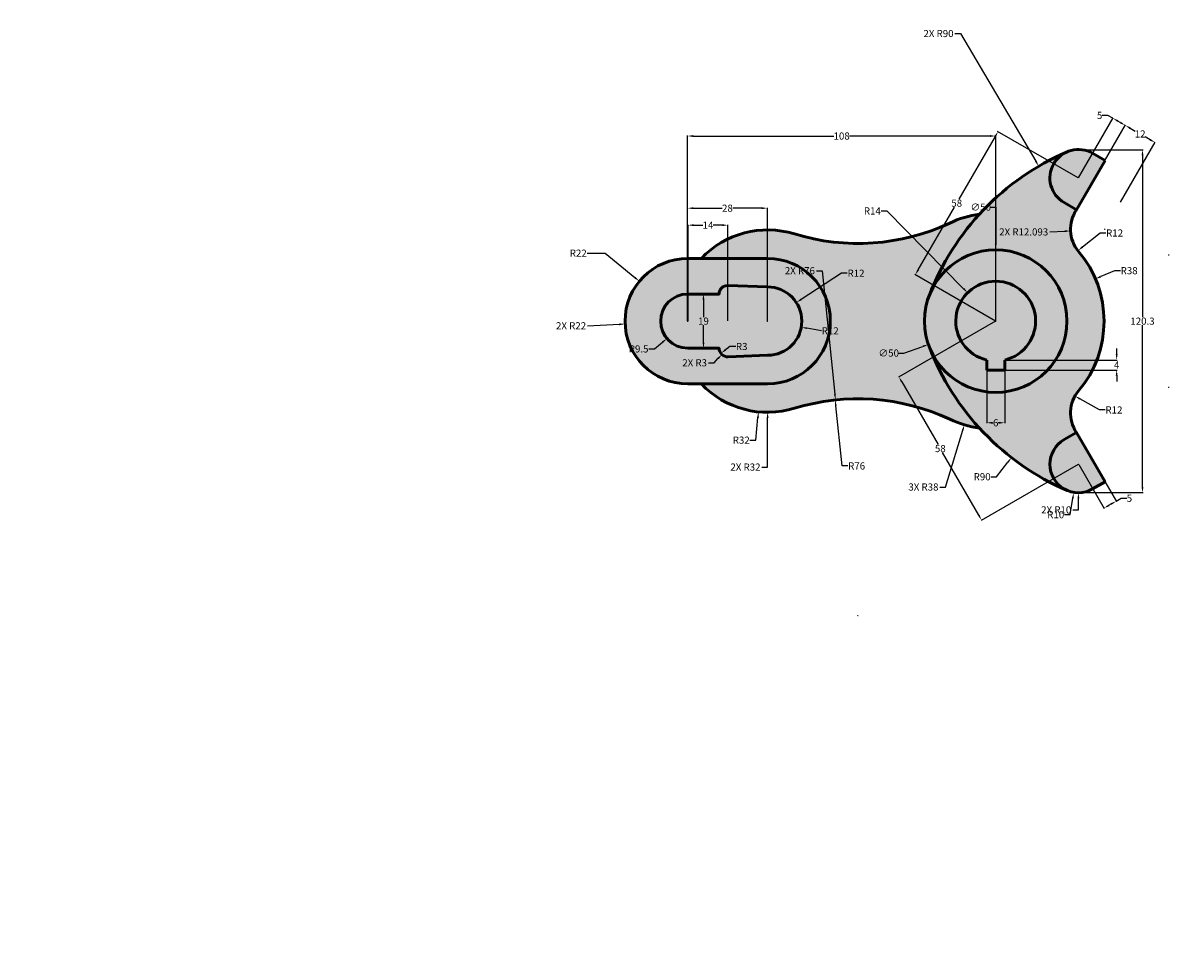
# Model space of a CAD drawing. Units: millimetres. Extents: x -3 to 399, y -3 to 324.
import ezdxf

# ---------------------------------------------------------------- set-up
doc = ezdxf.new("R2010")
doc.units = ezdxf.units.MM
doc.header["$MEASUREMENT"] = 0
for name, color, linetype, lineweight in [('Dimension', 120, 'Continuous', 25), ('M-CONS', 8, 'Continuous', 13), ('M-OUTL', 1, 'Continuous', 50)]:
    doc.layers.add(name, color=color, linetype=linetype, lineweight=lineweight)
doc.layers.add('M-HATC', color=9, linetype='Continuous', lineweight=18, true_color=0xc7c8ca)
doc.styles.get("Standard").update_dxf_attribs({"font": 'arial.ttf'})
doc.dimstyles.get("Standard").update_dxf_attribs({"dimtxt": 2.5, "dimasz": 2, "dimexe": 0.18, "dimexo": 0.0625, "dimgap": 0.09, "dimtad": 0, "dimtih": 1, "dimtoh": 1, "dimdec": 0, "dimzin": 0, "dimdsep": 46, "dimtxsty": 'Standard', "dimcen": 0.09, "dimadec": 0, "dimazin": 0, "dimtfac": 1, "dimtdec": 0, "dimtofl": 0, "dimtmove": 0, "dimatfit": 3, "dimfxl": 1, "dimtolj": 1, "dimtzin": 0, "dimarcsym": 0})

# ---------------------------------------------------------------- blocks, each defined once
blk = doc.blocks.new('*D1')
at = {"layer": 'Defpoints', "color": 0, "transparency": 16777216}
for p in [(213.19, 233.77), (230.17, 219.78)]:
    blk.add_point(p, dxfattribs=at)
at = {"layer": 'Dimension', "color": 0, "lineweight": -2, "transparency": 16777216}
for p, q in [((194.83, 243.63), (201.21, 243.63)), ((201.21, 243.63), (211.64, 235.04)), ((230.08, 219.78), (230.26, 219.78)), ((230.17, 219.69), (230.17, 219.87))]:
    blk.add_line(p, q, dxfattribs=at)
at = {"layer": 'Dimension', "color": 0, "transparency": 16777216}
blk.add_solid([(211.86, 235.3), (211.43, 234.78), (213.19, 233.77)], dxfattribs=at)
at = {"layer": 'Dimension', "color": 0, "transparency": 16777216, "insert": (191.77, 243.63), "char_height": 2.5, "attachment_point": 5}
blk.add_mtext('\\A1;R22', dxfattribs=at)
blk = doc.blocks.new('*D2')
at = {"layer": 'Defpoints', "color": 0, "transparency": 16777216}
for p in [(235.67, 229.28), (235.67, 210.28), (235.67, 210.28)]:
    blk.add_point(p, dxfattribs=at)
at = {"layer": 'Dimension', "color": 0, "lineweight": -2, "transparency": 16777216}
for p, q in [((235.73, 229.28), (235.85, 229.28)), ((235.67, 227.28), (235.67, 221.15)), ((235.67, 212.28), (235.67, 218.41)), ((235.73, 210.28), (235.85, 210.28))]:
    blk.add_line(p, q, dxfattribs=at)
at = {"layer": 'Dimension', "color": 0, "transparency": 16777216}
for points in [[(235.34, 227.28), (236, 227.28), (235.67, 229.28)], [(235.34, 212.28), (236, 212.28), (235.67, 210.28)]]:
    blk.add_solid(points, dxfattribs=at)
at = {"layer": 'Dimension', "color": 0, "transparency": 16777216, "insert": (235.67, 219.78), "char_height": 2.5, "attachment_point": 5}
blk.add_mtext('\\A1;19', dxfattribs=at)
blk = doc.blocks.new('*D3')
at = {"layer": 'Defpoints', "color": 0, "transparency": 16777216}
for p in [(244.17, 210.28), (241.76, 208.49)]:
    blk.add_point(p, dxfattribs=at)
at = {"layer": 'Dimension', "color": 0, "lineweight": -2, "transparency": 16777216}
for p, q in [((244.97, 210.88), (243.37, 209.68)), ((246.97, 210.88), (244.97, 210.88))]:
    blk.add_line(p, q, dxfattribs=at)
at = {"layer": 'Dimension', "color": 0, "transparency": 16777216}
blk.add_solid([(243.17, 209.95), (243.57, 209.42), (241.76, 208.49)], dxfattribs=at)
at = {"layer": 'Dimension', "color": 0, "transparency": 16777216, "insert": (249.08, 210.88), "char_height": 2.5, "attachment_point": 5}
blk.add_mtext('\\A1;R3', dxfattribs=at)
blk = doc.blocks.new('*D4')
at = {"layer": 'Defpoints', "color": 0, "transparency": 16777216}
for p in [(258.17, 219.78), (254.98, 187.94)]:
    blk.add_point(p, dxfattribs=at)
at = {"layer": 'Dimension', "color": 0, "lineweight": -2, "transparency": 16777216}
for p, q in [((258.08, 219.78), (258.26, 219.78)), ((258.17, 219.69), (258.17, 219.87)), ((253.99, 178.03), (254.78, 185.95)), ((251.99, 178.03), (253.99, 178.03))]:
    blk.add_line(p, q, dxfattribs=at)
at = {"layer": 'Dimension', "color": 0, "transparency": 16777216}
blk.add_solid([(254.45, 185.98), (255.12, 185.92), (254.98, 187.94)], dxfattribs=at)
at = {"layer": 'Dimension', "color": 0, "transparency": 16777216, "insert": (248.93, 178.03), "char_height": 2.5, "attachment_point": 5}
blk.add_mtext('\\A1;R32', dxfattribs=at)
blk = doc.blocks.new('*D5')
at = {"layer": 'Defpoints', "color": 0, "transparency": 16777216}
for p in [(258.08, 259.41), (230.08, 219.78), (258.08, 219.78)]:
    blk.add_point(p, dxfattribs=at)
at = {"layer": 'Dimension', "color": 0, "lineweight": -2, "transparency": 16777216}
for p, q in [((230.08, 219.84), (230.08, 259.59)), ((232.08, 259.41), (242.18, 259.41)), ((256.08, 259.41), (245.98, 259.41)), ((258.08, 219.84), (258.08, 259.59))]:
    blk.add_line(p, q, dxfattribs=at)
at = {"layer": 'Dimension', "color": 0, "transparency": 16777216}
for points in [[(232.08, 259.74), (232.08, 259.07), (230.08, 259.41)], [(256.08, 259.74), (256.08, 259.07), (258.08, 259.41)]]:
    blk.add_solid(points, dxfattribs=at)
at = {"layer": 'Dimension', "color": 0, "transparency": 16777216, "insert": (244.08, 259.41), "char_height": 2.5, "attachment_point": 5}
blk.add_mtext('\\A1;28', dxfattribs=at)
blk = doc.blocks.new('*D6')
at = {"layer": 'Defpoints', "color": 0, "transparency": 16777216}
for p in [(244.26, 253.44), (230.26, 219.78), (244.26, 219.78)]:
    blk.add_point(p, dxfattribs=at)
at = {"layer": 'Dimension', "color": 0, "lineweight": -2, "transparency": 16777216}
for p, q in [((230.26, 219.84), (230.26, 253.62)), ((232.26, 253.44), (235.5, 253.44)), ((242.26, 253.44), (239.02, 253.44)), ((244.26, 219.84), (244.26, 253.62))]:
    blk.add_line(p, q, dxfattribs=at)
at = {"layer": 'Dimension', "color": 0, "transparency": 16777216}
for points in [[(232.26, 253.78), (232.26, 253.11), (230.26, 253.44)], [(242.26, 253.78), (242.26, 253.11), (244.26, 253.44)]]:
    blk.add_solid(points, dxfattribs=at)
at = {"layer": 'Dimension', "color": 0, "transparency": 16777216, "insert": (237.26, 253.44), "char_height": 2.5, "attachment_point": 5}
blk.add_mtext('\\A1;14', dxfattribs=at)
blk = doc.blocks.new('*D7')
at = {"layer": 'Defpoints', "color": 0, "transparency": 16777216}
for p in [(338.17, 284.73), (230.08, 219.78), (338.17, 219.78)]:
    blk.add_point(p, dxfattribs=at)
at = {"layer": 'Dimension', "color": 0, "lineweight": -2, "transparency": 16777216}
for p, q in [((230.08, 219.84), (230.08, 284.91)), ((232.08, 284.73), (281.39, 284.73)), ((336.17, 284.73), (286.86, 284.73)), ((338.17, 219.84), (338.17, 284.91))]:
    blk.add_line(p, q, dxfattribs=at)
at = {"layer": 'Dimension', "color": 0, "transparency": 16777216}
for points in [[(232.08, 285.07), (232.08, 284.4), (230.08, 284.73)], [(336.17, 285.07), (336.17, 284.4), (338.17, 284.73)]]:
    blk.add_solid(points, dxfattribs=at)
at = {"layer": 'Dimension', "color": 0, "transparency": 16777216, "insert": (284.13, 284.73), "char_height": 2.5, "attachment_point": 5}
blk.add_mtext('\\A1;108', dxfattribs=at)
blk = doc.blocks.new('*D8')
at = {"layer": 'Defpoints', "color": 0, "transparency": 16777216}
for p in [(338.99, 286.28), (367.17, 270.01), (338.17, 219.78)]:
    blk.add_point(p, dxfattribs=at)
at = {"layer": 'Dimension', "color": 0, "lineweight": -2, "transparency": 16777216}
for p, q in [((367.12, 270.04), (338.83, 286.37)), ((337.99, 284.55), (325.28, 262.53)), ((310.99, 237.78), (323.7, 259.8)), ((338.12, 219.81), (309.83, 236.14))]:
    blk.add_line(p, q, dxfattribs=at)
at = {"layer": 'Dimension', "color": 0, "transparency": 16777216}
for points in [[(337.7, 284.72), (338.28, 284.38), (338.99, 286.28)], [(310.7, 237.95), (311.28, 237.62), (309.99, 236.05)]]:
    blk.add_solid(points, dxfattribs=at)
at = {"layer": 'Dimension', "color": 0, "transparency": 16777216, "insert": (324.49, 261.17), "char_height": 2.5, "attachment_point": 5}
blk.add_mtext('\\A1;58', dxfattribs=at)
blk = doc.blocks.new('*D9')
at = {"layer": 'Defpoints', "color": 0, "transparency": 16777216}
for p in [(281.87, 192.11), (289.85, 116.53)]:
    blk.add_point(p, dxfattribs=at)
at = {"layer": 'Dimension', "color": 0, "lineweight": -2, "transparency": 16777216}
for p, q in [((284.31, 168.97), (282.08, 190.12)), ((286.31, 168.97), (284.31, 168.97))]:
    blk.add_line(p, q, dxfattribs=at)
at = {"layer": 'Dimension', "color": 0, "transparency": 16777216}
blk.add_solid([(282.41, 190.16), (281.75, 190.09), (281.87, 192.11)], dxfattribs=at)
at = {"layer": 'Dimension', "color": 0, "transparency": 16777216, "insert": (289.39, 168.97), "char_height": 2.5, "attachment_point": 5}
blk.add_mtext('\\A1;R76', dxfattribs=at)
blk = doc.blocks.new('*D10')
at = {"layer": 'Defpoints', "color": 0, "transparency": 16777216}
for p in [(338.17, 219.78), (367.17, 169.55), (333.23, 149.95)]:
    blk.add_point(p, dxfattribs=at)
at = {"layer": 'Dimension', "color": 0, "lineweight": -2, "transparency": 16777216}
for p, q in [((338.12, 219.75), (304.07, 200.09)), ((305.23, 198.45), (317.94, 176.44)), ((332.23, 151.69), (319.51, 173.7)), ((367.12, 169.52), (333.07, 149.86))]:
    blk.add_line(p, q, dxfattribs=at)
at = {"layer": 'Dimension', "color": 0, "transparency": 16777216}
for points in [[(305.51, 198.62), (304.94, 198.29), (304.23, 200.18)], [(332.51, 151.85), (331.94, 151.52), (333.23, 149.95)]]:
    blk.add_solid(points, dxfattribs=at)
at = {"layer": 'Dimension', "color": 0, "transparency": 16777216, "insert": (318.73, 175.07), "char_height": 2.5, "attachment_point": 5}
blk.add_mtext('\\A1;58', dxfattribs=at)
blk = doc.blocks.new('*D11')
at = {"layer": 'Defpoints', "color": 0, "transparency": 16777216}
for p in [(398.88, 243), (343.69, 171.91)]:
    blk.add_point(p, dxfattribs=at)
at = {"layer": 'Dimension', "color": 0, "lineweight": -2, "transparency": 16777216}
for p, q in [((398.79, 243), (398.97, 243)), ((398.88, 242.91), (398.88, 243.09)), ((338.48, 165.19), (342.47, 170.33)), ((336.48, 165.19), (338.48, 165.19))]:
    blk.add_line(p, q, dxfattribs=at)
at = {"layer": 'Dimension', "color": 0, "transparency": 16777216}
blk.add_solid([(342.2, 170.53), (342.73, 170.12), (343.69, 171.91)], dxfattribs=at)
at = {"layer": 'Dimension', "color": 0, "transparency": 16777216, "insert": (333.41, 165.19), "char_height": 2.5, "attachment_point": 5}
blk.add_mtext('\\A1;R90', dxfattribs=at)
blk = doc.blocks.new('*D12')
at = {"layer": 'Defpoints', "color": 0, "transparency": 16777216}
for p in [(361.79, 227.98), (314.55, 211.59)]:
    blk.add_point(p, dxfattribs=at)
at = {"layer": 'Dimension', "color": 0, "lineweight": -2, "transparency": 16777216}
for p, q in [((338.08, 219.78), (338.26, 219.78)), ((338.17, 219.69), (338.17, 219.87)), ((305.89, 208.58), (312.66, 210.93)), ((303.89, 208.58), (305.89, 208.58))]:
    blk.add_line(p, q, dxfattribs=at)
at = {"layer": 'Dimension', "color": 0, "transparency": 16777216}
blk.add_solid([(312.55, 211.24), (312.77, 210.62), (314.55, 211.59)], dxfattribs=at)
at = {"layer": 'Dimension', "color": 0, "transparency": 16777216, "insert": (300.65, 208.58), "char_height": 2.5, "attachment_point": 5}
blk.add_mtext('\\A1;∅50', dxfattribs=at)
blk = doc.blocks.new('*D13')
at = {"layer": 'Defpoints', "color": 0, "transparency": 16777216}
for p in [(268.24, 226.31), (258.17, 219.78)]:
    blk.add_point(p, dxfattribs=at)
at = {"layer": 'Dimension', "color": 0, "lineweight": -2, "transparency": 16777216}
for p, q in [((284.11, 236.59), (269.92, 227.39)), ((286.11, 236.59), (284.11, 236.59)), ((258.08, 219.78), (258.26, 219.78)), ((258.17, 219.69), (258.17, 219.87))]:
    blk.add_line(p, q, dxfattribs=at)
at = {"layer": 'Dimension', "color": 0, "transparency": 16777216}
blk.add_solid([(269.74, 227.67), (270.1, 227.11), (268.24, 226.31)], dxfattribs=at)
at = {"layer": 'Dimension', "color": 0, "transparency": 16777216, "insert": (289.18, 236.59), "char_height": 2.5, "attachment_point": 5}
blk.add_mtext('\\A1;R12', dxfattribs=at)
blk = doc.blocks.new('*D14')
at = {"layer": 'Defpoints', "color": 0, "transparency": 16777216}
for p in [(328.33, 229.74), (338.17, 219.78)]:
    blk.add_point(p, dxfattribs=at)
at = {"layer": 'Dimension', "color": 0, "lineweight": -2, "transparency": 16777216}
for p, q in [((297.98, 258.44), (299.98, 258.44)), ((299.98, 258.44), (326.93, 231.16)), ((338.08, 219.78), (338.26, 219.78)), ((338.17, 219.69), (338.17, 219.87))]:
    blk.add_line(p, q, dxfattribs=at)
at = {"layer": 'Dimension', "color": 0, "transparency": 16777216}
blk.add_solid([(327.16, 231.4), (326.69, 230.93), (328.33, 229.74)], dxfattribs=at)
at = {"layer": 'Dimension', "color": 0, "transparency": 16777216, "insert": (294.91, 258.44), "char_height": 2.5, "attachment_point": 5}
blk.add_mtext('\\A1;R14', dxfattribs=at)
blk = doc.blocks.new('*D15')
at = {"layer": 'Defpoints', "color": 0, "transparency": 16777216}
for p in [(341.32, 206.14), (341.32, 202.63), (380.6, 202.63)]:
    blk.add_point(p, dxfattribs=at)
at = {"layer": 'Dimension', "color": 0, "lineweight": -2, "transparency": 16777216}
for p, q in [((380.6, 208.14), (380.6, 210.14)), ((341.38, 206.14), (380.78, 206.14)), ((341.38, 202.63), (380.78, 202.63)), ((380.6, 200.63), (380.6, 198.63))]:
    blk.add_line(p, q, dxfattribs=at)
at = {"layer": 'Dimension', "color": 0, "transparency": 16777216}
for points in [[(380.26, 208.14), (380.93, 208.14), (380.6, 206.14)], [(380.26, 200.63), (380.93, 200.63), (380.6, 202.63)]]:
    blk.add_solid(points, dxfattribs=at)
at = {"layer": 'Dimension', "color": 0, "transparency": 16777216, "insert": (380.6, 204.39), "char_height": 2.5, "attachment_point": 5}
blk.add_mtext('\\A1;4', dxfattribs=at)
blk = doc.blocks.new('*D16')
at = {"layer": 'Defpoints', "color": 0, "transparency": 16777216}
for p in [(335.02, 202.63), (341.32, 202.63), (341.32, 184.12)]:
    blk.add_point(p, dxfattribs=at)
at = {"layer": 'Dimension', "color": 0, "lineweight": -2, "transparency": 16777216}
for p, q in [((335.02, 202.57), (335.02, 183.94)), ((341.32, 202.57), (341.32, 183.94)), ((337.02, 184.12), (337.25, 184.12)), ((339.32, 184.12), (339.09, 184.12))]:
    blk.add_line(p, q, dxfattribs=at)
at = {"layer": 'Dimension', "color": 0, "transparency": 16777216}
for points in [[(337.02, 184.45), (337.02, 183.78), (335.02, 184.12)], [(339.32, 184.45), (339.32, 183.78), (341.32, 184.12)]]:
    blk.add_solid(points, dxfattribs=at)
at = {"layer": 'Dimension', "color": 0, "transparency": 16777216, "insert": (338.17, 184.12), "char_height": 2.5, "attachment_point": 5}
blk.add_mtext('\\A1;6', dxfattribs=at)
blk = doc.blocks.new('*D17')
at = {"layer": 'Defpoints', "color": 0, "transparency": 16777216}
for p in [(367.17, 169.55), (365.56, 159.68)]:
    blk.add_point(p, dxfattribs=at)
at = {"layer": 'Dimension', "color": 0, "lineweight": -2, "transparency": 16777216}
for p, q in [((367.08, 169.55), (367.26, 169.55)), ((367.17, 169.46), (367.17, 169.64)), ((364.29, 151.88), (365.24, 157.71)), ((362.29, 151.88), (364.29, 151.88))]:
    blk.add_line(p, q, dxfattribs=at)
at = {"layer": 'Dimension', "color": 0, "transparency": 16777216}
blk.add_solid([(364.91, 157.76), (365.57, 157.65), (365.56, 159.68)], dxfattribs=at)
at = {"layer": 'Dimension', "color": 0, "transparency": 16777216, "insert": (359.22, 151.88), "char_height": 2.5, "attachment_point": 5}
blk.add_mtext('\\A1;R10', dxfattribs=at)
blk = doc.blocks.new('*D18')
at = {"layer": 'Defpoints', "color": 0, "transparency": 16777216}
for p in [(367.26, 169.55), (371.52, 172.01), (380.41, 156.62)]:
    blk.add_point(p, dxfattribs=at)
at = {"layer": 'Dimension', "color": 0, "lineweight": -2, "transparency": 16777216}
for p, q in [((367.29, 169.5), (376.24, 154.01)), ((371.55, 171.96), (380.5, 156.47)), ((380.41, 156.62), (382.14, 157.62)), ((382.14, 157.62), (384.14, 157.62)), ((377.88, 155.16), (378.68, 155.62))]:
    blk.add_line(p, q, dxfattribs=at)
at = {"layer": 'Dimension', "color": 0, "transparency": 16777216}
for points in [[(377.71, 155.45), (378.04, 154.87), (376.15, 154.16)], [(378.51, 155.91), (378.84, 155.33), (380.41, 156.62)]]:
    blk.add_solid(points, dxfattribs=at)
at = {"layer": 'Dimension', "color": 0, "transparency": 16777216, "insert": (385.06, 157.62), "char_height": 2.5, "attachment_point": 5}
blk.add_mtext('\\A1;5', dxfattribs=at)
blk = doc.blocks.new('*D19')
at = {"layer": 'Defpoints', "color": 0, "transparency": 16777216}
for p in [(394.06, 282.43), (371.5, 267.51), (381.96, 261.47)]:
    blk.add_point(p, dxfattribs=at)
at = {"layer": 'Dimension', "color": 0, "lineweight": -2, "transparency": 16777216}
for p, q in [((371.53, 267.56), (383.69, 288.62)), ((385.33, 287.47), (387.08, 286.46)), ((381.99, 261.53), (394.15, 282.58)), ((392.33, 283.43), (390.58, 284.44))]:
    blk.add_line(p, q, dxfattribs=at)
at = {"layer": 'Dimension', "color": 0, "transparency": 16777216}
for points in [[(385.5, 287.76), (385.16, 287.18), (383.6, 288.47)], [(392.49, 283.72), (392.16, 283.14), (394.06, 282.43)]]:
    blk.add_solid(points, dxfattribs=at)
at = {"layer": 'Dimension', "color": 0, "transparency": 16777216, "insert": (388.83, 285.45), "char_height": 2.5, "attachment_point": 5}
blk.add_mtext('\\A1;12', dxfattribs=at)
blk = doc.blocks.new('*D20')
at = {"layer": 'Defpoints', "color": 0, "transparency": 16777216}
for p in [(379.27, 290.97), (367.17, 270.01), (371.5, 267.51)]:
    blk.add_point(p, dxfattribs=at)
at = {"layer": 'Dimension', "color": 0, "lineweight": -2, "transparency": 16777216}
for p, q in [((367.2, 270.06), (379.36, 291.12)), ((377.54, 291.97), (375.54, 291.97)), ((379.27, 290.97), (377.54, 291.97)), ((381.87, 289.47), (381, 289.97)), ((371.53, 267.56), (383.69, 288.62))]:
    blk.add_line(p, q, dxfattribs=at)
at = {"layer": 'Dimension', "color": 0, "transparency": 16777216}
for points in [[(381.17, 290.26), (380.83, 289.68), (379.27, 290.97)], [(382.03, 289.76), (381.7, 289.18), (383.6, 288.47)]]:
    blk.add_solid(points, dxfattribs=at)
at = {"layer": 'Dimension', "color": 0, "transparency": 16777216, "insert": (374.62, 291.97), "char_height": 2.5, "attachment_point": 5}
blk.add_mtext('\\A1;5', dxfattribs=at)
blk = doc.blocks.new('*D21')
at = {"layer": 'Defpoints', "color": 0, "transparency": 16777216}
for p in [(376.49, 252.04), (367.02, 244.52)]:
    blk.add_point(p, dxfattribs=at)
at = {"layer": 'Dimension', "color": 0, "lineweight": -2, "transparency": 16777216}
for p, q in [((374.8, 250.7), (368.59, 245.77)), ((376.8, 250.7), (374.8, 250.7))]:
    blk.add_line(p, q, dxfattribs=at)
at = {"layer": 'Dimension', "color": 0, "transparency": 16777216}
blk.add_solid([(368.38, 246.03), (368.79, 245.51), (367.02, 244.52)], dxfattribs=at)
at = {"layer": 'Dimension', "color": 0, "transparency": 16777216, "insert": (379.87, 250.7), "char_height": 2.5, "attachment_point": 5}
blk.add_mtext('\\A1;R12', dxfattribs=at)
blk = doc.blocks.new('*D22')
at = {"layer": 'Defpoints', "color": 0, "transparency": 16777216}
for p in [(373.15, 234.62), (338.17, 219.78)]:
    blk.add_point(p, dxfattribs=at)
at = {"layer": 'Dimension', "color": 0, "lineweight": -2, "transparency": 16777216}
for p, q in [((379.88, 237.48), (374.99, 235.4)), ((381.88, 237.48), (379.88, 237.48)), ((338.08, 219.78), (338.26, 219.78)), ((338.17, 219.69), (338.17, 219.87))]:
    blk.add_line(p, q, dxfattribs=at)
at = {"layer": 'Dimension', "color": 0, "transparency": 16777216}
blk.add_solid([(374.86, 235.71), (375.12, 235.1), (373.15, 234.62)], dxfattribs=at)
at = {"layer": 'Dimension', "color": 0, "transparency": 16777216, "insert": (384.96, 237.48), "char_height": 2.5, "attachment_point": 5}
blk.add_mtext('\\A1;R38', dxfattribs=at)
blk = doc.blocks.new('*D23')
at = {"layer": 'Defpoints', "color": 0, "transparency": 16777216}
for p in [(365.97, 193.49), (376.49, 187.52)]:
    blk.add_point(p, dxfattribs=at)
at = {"layer": 'Dimension', "color": 0, "lineweight": -2, "transparency": 16777216}
for p, q in [((374.58, 188.61), (367.71, 192.5)), ((376.58, 188.61), (374.58, 188.61))]:
    blk.add_line(p, q, dxfattribs=at)
at = {"layer": 'Dimension', "color": 0, "transparency": 16777216}
blk.add_solid([(367.88, 192.79), (367.55, 192.21), (365.97, 193.49)], dxfattribs=at)
at = {"layer": 'Dimension', "color": 0, "transparency": 16777216, "insert": (379.64, 188.61), "char_height": 2.5, "attachment_point": 5}
blk.add_mtext('\\A1;R12', dxfattribs=at)
blk = doc.blocks.new('*D24')
at = {"layer": 'Defpoints', "color": 0, "transparency": 16777216}
for p in [(368.41, 279.94), (389.65, 279.94), (368.41, 159.63)]:
    blk.add_point(p, dxfattribs=at)
at = {"layer": 'Dimension', "color": 0, "lineweight": -2, "transparency": 16777216}
for p, q in [((368.47, 279.94), (389.83, 279.94)), ((389.65, 277.94), (389.65, 221.15)), ((389.65, 161.63), (389.65, 218.41)), ((368.47, 159.63), (389.83, 159.63))]:
    blk.add_line(p, q, dxfattribs=at)
at = {"layer": 'Dimension', "color": 0, "transparency": 16777216}
for points in [[(389.32, 277.94), (389.98, 277.94), (389.65, 279.94)], [(389.32, 161.63), (389.98, 161.63), (389.65, 159.63)]]:
    blk.add_solid(points, dxfattribs=at)
at = {"layer": 'Dimension', "color": 0, "transparency": 16777216, "insert": (389.65, 219.78), "char_height": 2.5, "attachment_point": 5}
blk.add_mtext('\\A1;120.3', dxfattribs=at)
blk = doc.blocks.new('*D25')
at = {"layer": 'Defpoints', "color": 0, "transparency": 16777216}
for p in [(258.17, 219.78), (269.98, 217.65)]:
    blk.add_point(p, dxfattribs=at)
at = {"layer": 'Dimension', "color": 0, "lineweight": -2, "transparency": 16777216}
for p, q in [((258.08, 219.78), (258.26, 219.78)), ((258.17, 219.69), (258.17, 219.87)), ((277.06, 216.37), (271.95, 217.29))]:
    blk.add_line(p, q, dxfattribs=at)
at = {"layer": 'Dimension', "color": 0, "transparency": 16777216}
blk.add_solid([(272.01, 217.62), (271.89, 216.97), (269.98, 217.65)], dxfattribs=at)
at = {"layer": 'Dimension', "color": 0, "transparency": 16777216, "insert": (280.13, 216.37), "char_height": 2.5, "attachment_point": 5}
blk.add_mtext('\\A1;R12', dxfattribs=at)
blk = doc.blocks.new('*D26')
at = {"layer": 'Defpoints', "color": 0, "transparency": 16777216}
for p in [(244.17, 210.28), (242.13, 208.09)]:
    blk.add_point(p, dxfattribs=at)
at = {"layer": 'Dimension', "color": 0, "lineweight": -2, "transparency": 16777216}
for p, q in [((244.08, 210.28), (244.26, 210.28)), ((244.17, 210.19), (244.17, 210.37)), ((237.4, 205.16), (239.4, 205.16)), ((239.4, 205.16), (240.76, 206.62))]:
    blk.add_line(p, q, dxfattribs=at)
at = {"layer": 'Dimension', "color": 0, "transparency": 16777216}
blk.add_solid([(240.52, 206.85), (241.01, 206.39), (242.13, 208.09)], dxfattribs=at)
at = {"layer": 'Dimension', "color": 0, "transparency": 16777216, "insert": (232.59, 205.16), "char_height": 2.5, "attachment_point": 5}
blk.add_mtext('\\A1;2X R3', dxfattribs=at)
blk = doc.blocks.new('*D27')
at = {"layer": 'Defpoints', "color": 0, "transparency": 16777216}
for p in [(208.19, 218.76), (230.17, 219.78)]:
    blk.add_point(p, dxfattribs=at)
at = {"layer": 'Dimension', "color": 0, "lineweight": -2, "transparency": 16777216}
for p, q in [((195.01, 218.15), (206.2, 218.67)), ((230.08, 219.78), (230.26, 219.78)), ((230.17, 219.69), (230.17, 219.87))]:
    blk.add_line(p, q, dxfattribs=at)
at = {"layer": 'Dimension', "color": 0, "transparency": 16777216}
blk.add_solid([(206.18, 219), (206.21, 218.33), (208.19, 218.76)], dxfattribs=at)
at = {"layer": 'Dimension', "color": 0, "transparency": 16777216, "insert": (189.24, 218.15), "char_height": 2.5, "attachment_point": 5}
blk.add_mtext('\\A1;2X R22', dxfattribs=at)
blk = doc.blocks.new('*D28')
at = {"layer": 'Defpoints', "color": 0, "transparency": 16777216}
for p in [(258.17, 219.78), (258.17, 187.78)]:
    blk.add_point(p, dxfattribs=at)
at = {"layer": 'Dimension', "color": 0, "lineweight": -2, "transparency": 16777216}
for p, q in [((258.08, 219.78), (258.26, 219.78)), ((258.17, 219.69), (258.17, 219.87)), ((258.17, 168.58), (258.17, 185.78)), ((256.17, 168.58), (258.17, 168.58))]:
    blk.add_line(p, q, dxfattribs=at)
at = {"layer": 'Dimension', "color": 0, "transparency": 16777216}
blk.add_solid([(257.84, 185.78), (258.5, 185.78), (258.17, 187.78)], dxfattribs=at)
at = {"layer": 'Dimension', "color": 0, "transparency": 16777216, "insert": (250.4, 168.58), "char_height": 2.5, "attachment_point": 5}
blk.add_mtext('\\A1;2X R32', dxfattribs=at)
blk = doc.blocks.new('*D29')
at = {"layer": 'Defpoints', "color": 0, "transparency": 16777216}
for p in [(281.99, 192.12), (289.85, 116.53)]:
    blk.add_point(p, dxfattribs=at)
at = {"layer": 'Dimension', "color": 0, "lineweight": -2, "transparency": 16777216}
for p, q in [((275.27, 237.48), (277.27, 237.48)), ((277.27, 237.48), (281.78, 194.11)), ((289.85, 116.44), (289.85, 116.62)), ((289.76, 116.53), (289.94, 116.53))]:
    blk.add_line(p, q, dxfattribs=at)
at = {"layer": 'Dimension', "color": 0, "transparency": 16777216}
blk.add_solid([(282.11, 194.15), (281.45, 194.08), (281.99, 192.12)], dxfattribs=at)
at = {"layer": 'Dimension', "color": 0, "transparency": 16777216, "insert": (269.49, 237.48), "char_height": 2.5, "attachment_point": 5}
blk.add_mtext('\\A1;2X R76', dxfattribs=at)
blk = doc.blocks.new('*D30')
at = {"layer": 'Defpoints', "color": 0, "transparency": 16777216}
for p in [(353.25, 274.14), (398.88, 196.56)]:
    blk.add_point(p, dxfattribs=at)
at = {"layer": 'Dimension', "color": 0, "lineweight": -2, "transparency": 16777216}
for p, q in [((323.88, 320.69), (325.88, 320.69)), ((325.88, 320.69), (352.24, 275.86)), ((398.79, 196.56), (398.97, 196.56)), ((398.88, 196.47), (398.88, 196.65))]:
    blk.add_line(p, q, dxfattribs=at)
at = {"layer": 'Dimension', "color": 0, "transparency": 16777216}
blk.add_solid([(352.53, 276.03), (351.95, 275.7), (353.25, 274.14)], dxfattribs=at)
at = {"layer": 'Dimension', "color": 0, "transparency": 16777216, "insert": (318.1, 320.69), "char_height": 2.5, "attachment_point": 5}
blk.add_mtext('\\A1;2X R90', dxfattribs=at)
blk = doc.blocks.new('*D31')
at = {"layer": 'Defpoints', "color": 0, "transparency": 16777216}
for p in [(367.17, 169.55), (367.17, 159.55)]:
    blk.add_point(p, dxfattribs=at)
at = {"layer": 'Dimension', "color": 0, "lineweight": -2, "transparency": 16777216}
for p, q in [((367.08, 169.55), (367.26, 169.55)), ((367.17, 169.46), (367.17, 169.64)), ((367.17, 153.55), (367.17, 157.55)), ((365.17, 153.55), (367.17, 153.55))]:
    blk.add_line(p, q, dxfattribs=at)
at = {"layer": 'Dimension', "color": 0, "transparency": 16777216}
blk.add_solid([(366.84, 157.55), (367.5, 157.55), (367.17, 159.55)], dxfattribs=at)
at = {"layer": 'Dimension', "color": 0, "transparency": 16777216, "insert": (359.39, 153.55), "char_height": 2.5, "attachment_point": 5}
blk.add_mtext('\\A1;2X R10', dxfattribs=at)
blk = doc.blocks.new('*D32')
at = {"layer": 'Defpoints', "color": 0, "transparency": 16777216}
for p in [(364.42, 251.44), (376.49, 252.04)]:
    blk.add_point(p, dxfattribs=at)
at = {"layer": 'Dimension', "color": 0, "lineweight": -2, "transparency": 16777216}
for p, q in [((357.17, 251.08), (362.42, 251.34)), ((376.4, 252.04), (376.58, 252.04)), ((376.49, 251.95), (376.49, 252.13))]:
    blk.add_line(p, q, dxfattribs=at)
at = {"layer": 'Dimension', "color": 0, "transparency": 16777216}
blk.add_solid([(362.4, 251.67), (362.43, 251.01), (364.42, 251.44)], dxfattribs=at)
at = {"layer": 'Dimension', "color": 0, "transparency": 16777216, "insert": (347.99, 251.08), "char_height": 2.5, "attachment_point": 5}
blk.add_mtext('\\A1;2X R12.093', dxfattribs=at)
blk = doc.blocks.new('*D33')
at = {"layer": 'Defpoints', "color": 0, "transparency": 16777216}
for p in [(338.17, 219.78), (327.18, 183.41)]:
    blk.add_point(p, dxfattribs=at)
at = {"layer": 'Dimension', "color": 0, "lineweight": -2, "transparency": 16777216}
for p, q in [((338.08, 219.78), (338.26, 219.78)), ((338.17, 219.69), (338.17, 219.87)), ((320.58, 161.58), (326.6, 181.49)), ((318.58, 161.58), (320.58, 161.58))]:
    blk.add_line(p, q, dxfattribs=at)
at = {"layer": 'Dimension', "color": 0, "transparency": 16777216}
blk.add_solid([(326.28, 181.59), (326.92, 181.4), (327.18, 183.41)], dxfattribs=at)
at = {"layer": 'Dimension', "color": 0, "transparency": 16777216, "insert": (312.82, 161.58), "char_height": 2.5, "attachment_point": 5}
blk.add_mtext('\\A1;3X R38', dxfattribs=at)
blk = doc.blocks.new('*D34')
at = {"layer": 'Defpoints', "color": 0, "transparency": 16777216}
for p in [(338.17, 244.78), (338.17, 194.78)]:
    blk.add_point(p, dxfattribs=at)
at = {"layer": 'Dimension', "color": 0, "lineweight": -2, "transparency": 16777216}
for p, q in [((336.17, 259.78), (338.17, 259.78)), ((338.17, 259.78), (338.17, 246.78)), ((338.08, 219.78), (338.26, 219.78)), ((338.17, 219.69), (338.17, 219.87))]:
    blk.add_line(p, q, dxfattribs=at)
at = {"layer": 'Dimension', "color": 0, "transparency": 16777216}
blk.add_solid([(338.5, 246.78), (337.84, 246.78), (338.17, 244.78)], dxfattribs=at)
at = {"layer": 'Dimension', "color": 0, "transparency": 16777216, "insert": (332.93, 259.78), "char_height": 2.5, "attachment_point": 5}
blk.add_mtext('\\A1;∅50', dxfattribs=at)
blk = doc.blocks.new('*D35')
at = {"layer": 'Defpoints', "color": 0, "transparency": 16777216}
for p in [(230.17, 219.78), (222.88, 213.69)]:
    blk.add_point(p, dxfattribs=at)
at = {"layer": 'Dimension', "color": 0, "lineweight": -2, "transparency": 16777216}
for p, q in [((230.08, 219.78), (230.26, 219.78)), ((230.17, 219.69), (230.17, 219.87)), ((216.51, 210.03), (218.51, 210.03)), ((218.51, 210.03), (221.35, 212.4))]:
    blk.add_line(p, q, dxfattribs=at)
at = {"layer": 'Dimension', "color": 0, "transparency": 16777216}
blk.add_solid([(221.14, 212.66), (221.56, 212.15), (222.88, 213.69)], dxfattribs=at)
at = {"layer": 'Dimension', "color": 0, "transparency": 16777216, "insert": (212.94, 210.03), "char_height": 2.5, "attachment_point": 5}
blk.add_mtext('\\A1;R9.5', dxfattribs=at)

msp = doc.modelspace()

# ---------------------------------------------------------------- hatches: boundary and pattern name
at = {"layer": 'M-HATC'}
h = msp.add_hatch(color=256, dxfattribs=at)
h.dxf.hatch_style = 1
h.paths.add_polyline_path([(258.1701, 241.7814), (230.1701, 241.7814, 1), (230.1701, 197.7814), (258.1701, 197.7814, 1)])
h.paths.add_polyline_path([(230.1701, 229.2814), (241.1701, 229.2814, -0.41421356), (244.1701, 232.2814), (258.1701, 231.7814, -1), (258.1701, 207.7814), (244.3841, 207.289, -0.43528364), (241.1701, 210.2814), (230.1701, 210.2814, -1)], flags=16)
h.paths.add_polyline_path([(332.5192, 257.3589, 0.0722478), (322.0618, 254.1982, -0.18595349), (267.5553, 250.3741, 0.28496275), (234.9322, 241.7814), (258.1701, 241.7814, -1), (258.1701, 197.7814), (234.9322, 197.7814, 0.28496275), (267.5553, 189.1886, -0.18595349), (322.0618, 185.3645, 0.0722478), (332.5192, 182.2039, -0.09437457), (314.8192, 210.8519, -0.091566), (313.1701, 219.7814, -0.091566), (314.8192, 228.7108, -0.09437457)])
h.paths.add_polyline_path([(366.5002, 258.8506), (362.1701, 261.3506, -0.61668719), (363.2061, 279.1916, 0.20217753), (314.8192, 228.7108, -0.83223003), (363.1701, 219.7814, -0.83223003), (314.8192, 210.8519, 0.20217753), (363.2061, 160.3711, -0.61668719), (362.1701, 178.2121), (366.5002, 180.7121, -0.33687946), (367.2558, 195.3269, 0.36452561), (367.2558, 244.2358, -0.33687946)])
h = msp.add_hatch(color=256, dxfattribs=at)
h.dxf.hatch_style = 1
h.paths.add_polyline_path([(313.1701, 219.7814, 1), (363.1701, 219.7814, 1)])
h.paths.add_polyline_path([(341.3201, 206.1403), (341.3201, 202.6314), (338.1701, 202.6314), (335.0201, 202.6314), (335.0201, 206.1403, -8.77492784)], flags=16)
h.paths.add_polyline_path([(376.5002, 276.1711), (372.1701, 278.6711, 1), (362.1701, 261.3506), (366.5002, 258.8506)])
h.paths.add_polyline_path([(366.5002, 180.7121), (362.1701, 178.2121, 1), (372.1701, 160.8916), (376.5002, 163.3916)])
h.paths.add_polyline_path([(258.1701, 231.7814), (244.1701, 232.2814, 0.41421356), (241.1701, 229.2814), (230.1701, 229.2814, 1), (230.1701, 210.2814), (241.1701, 210.2814, 0.43528364), (244.3841, 207.289), (258.1701, 207.7814, 1)])
h = msp.add_hatch(color=256, dxfattribs=at)
h.dxf.hatch_style = 1
h.paths.add_polyline_path([(335.0201, 206.1403), (335.0201, 202.6314), (338.1701, 202.6314), (341.3201, 202.6314), (341.3201, 206.1403, 8.77492784)])

# ---------------------------------------------------------------- linework, layer by layer
at = {"layer": 'M-CONS'}
msp.add_arc((0, 0), 3, 0, 0, dxfattribs=at)
msp.add_arc((0, 0), 3, 0, 0, dxfattribs=at)
msp.add_arc((0, 0), 3, 0, 0, dxfattribs=at)
msp.add_arc((0, 0), 3, 0, 0, dxfattribs=at)
at = {"layer": 'M-OUTL'}
for p, q in [((372.1701, 278.6711), (376.5002, 276.1711)), ((366.5002, 258.8506), (376.5002, 276.1711)), ((362.1701, 261.3506), (366.5002, 258.8506)), ((230.1701, 241.7814), (258.1701, 241.7814)), ((244.1701, 232.2814), (258.1701, 231.7814)), ((244.3841, 207.289), (258.1701, 207.7814)), ((335.0201, 206.1403), (335.0201, 202.6314)), ((341.3201, 206.1403), (341.3201, 202.6314)), ((335.0201, 202.6314), (338.1701, 202.6314)), ((335.0201, 202.6314), (338.1701, 202.6314)), ((338.1701, 202.6314), (341.3201, 202.6314)), ((230.1701, 197.7814), (258.1701, 197.7814)), ((362.1701, 178.2121), (366.5002, 180.7121)), ((366.5002, 180.7121), (376.5002, 163.3916)), ((372.1701, 160.8916), (376.5002, 163.3916))]:
    msp.add_line(p, q, dxfattribs=at)
for points in [[(230.1701, 229.2814), (241.1701, 229.2814, -0.41421356), (244.1701, 232.2814, -0.41421356)], [(230.1701, 210.2814), (241.1701, 210.2814, 0.43528364), (244.3841, 207.289)]]:
    msp.add_lwpolyline(points, format="xyb", dxfattribs=at)
msp.add_circle((338.1701, 219.7814), 25, dxfattribs=at)
for centre, radius, start, end in [((398.8824, 196.5648), 90, 113.353588, 159.072975), ((367.1701, 270.0108), 10, 60, 240), ((338.1701, 219.7814), 38, 98.552023, 115.081279), ((376.4929, 252.0403), 12.0927, 145.724374, 219.984482), ((289.8451, 323.032), 76, 252.945151, 295.081279), ((258.1701, 219.7814), 32, 72.945151, 136.567463), ((230.1701, 219.7814), 22, 90, 270), ((258.1701, 219.7814), 22, 270, 90), ((338.1701, 219.7814), 38, 319.876874, 40.123126), ((338.1701, 219.7814), 14, 283.002878, 256.997122), ((230.1701, 219.7814), 9.5, 90, 270), ((258.1701, 219.7814), 12, 270, 90), ((398.8824, 242.998), 90, 200.927025, 246.646412), ((258.1701, 219.7814), 32, 223.432537, 287.054849), ((376.4929, 187.5224), 12.0927, 140.015518, 214.275626), ((289.8451, 116.5307), 76, 64.918721, 107.054849), ((338.1701, 219.7814), 38, 244.918721, 261.447977), ((367.1701, 169.5519), 10, 120, 300)]:
    msp.add_arc(centre, radius, start, end, dxfattribs=at)

# ---------------------------------------------------------------- dimensions: what is measured, and where the dimension line sits
at = {"layer": 'Dimension'}
for center, mpoint, text, override, picture, middle in [((398.8824, 196.5648), (353.2528, 274.1401), '2X <>', {"dimdec": 0, "dimlfac": 1, "dimrnd": 0, "dimzin": 0, "dimdsep": 46, "dimlunit": 2}, '*D30', (318.0953, 320.6854)), ((376.4929, 252.0403), (364.4152, 251.438), '2X <>', {"dimdec": 3, "dimlfac": 1, "dimrnd": 0, "dimzin": 0, "dimdsep": 46, "dimlunit": 2}, '*D32', (357.1686, 251.0766)), ((289.8451, 116.5307), (281.9872, 192.1234), '2X <>', {"dimdec": 0, "dimlfac": 1, "dimrnd": 0, "dimzin": 0, "dimdsep": 46, "dimlunit": 2}, '*D29', (269.4892, 237.479)), ((230.1701, 219.7814), (208.1938, 218.7602), '2X <>', {"dimdec": 0, "dimlfac": 1, "dimrnd": 0, "dimzin": 0, "dimdsep": 46, "dimlunit": 2}, '*D27', (195.008, 218.1475)), ((258.1701, 219.7814), (258.17, 187.7814), '2X <>', {"dimdec": 0, "dimlfac": 1, "dimrnd": 0, "dimzin": 0, "dimdsep": 46, "dimlunit": 2}, '*D28', (250.3987, 168.5814)), ((338.1701, 219.7814), (327.1761, 183.4065), '3X <>', {"dimdec": 0, "dimlfac": 1, "dimrnd": 0, "dimzin": 0, "dimdsep": 46, "dimlunit": 2}, '*D33', (312.8153, 161.5815)), ((367.1701, 169.5519), (367.17, 159.5519), '2X <>', {"dimdec": 0, "dimlfac": 1, "dimrnd": 0, "dimzin": 0, "dimdsep": 46, "dimlunit": 2}, '*D31', (359.3901, 153.5519))]:
    dim = msp.add_radius_dim(center=center, mpoint=mpoint, text=text, dimstyle='Standard', override=override, dxfattribs=at)
    dim.commit()
    dim.dimension.update_dxf_attribs({"geometry": picture, "text_midpoint": middle, "dimtype": 164})
for p1, p2, distance, picture, middle in [((371.5002, 267.5108), (367.1701, 270.0108), -24.1986, '*D20', (374.6186, 291.9675)), ((338.1701, 219.7814), (367.1701, 270.0108), 32.5409, '*D8', (324.4888, 261.1666)), ((371.5002, 267.5108), (381.961, 261.4713), 24.1986, '*D19', (388.8299, 285.4477)), ((338.1701, 219.7814), (367.1701, 169.5519), -39.1953, '*D10', (318.726, 175.069)), ((367.2601, 169.5519), (371.5227, 172.0129), -17.7709, '*D18', (385.059, 157.6228))]:
    dim = msp.add_aligned_dim(p1=p1, p2=p2, distance=distance, dimstyle='Standard', override={"dimclrd": 0, "dimclre": 0, "dimclrt": 0}, dxfattribs=at)
    dim.commit()
    dim.dimension.update_dxf_attribs({"geometry": picture, "text_midpoint": middle})
for base, p1, p2, picture, middle in [((338.1701, 284.7322), (230.0801, 219.7814), (338.1701, 219.7814), '*D7', (284.1251, 284.7322)), ((258.0801, 259.4069), (230.0801, 219.7814), (258.0801, 219.7814), '*D5', (244.0801, 259.4069)), ((244.2601, 253.4436), (230.2601, 219.7814), (244.2601, 219.7814), '*D6', (237.2601, 253.4436))]:
    dim = msp.add_linear_dim(base=base, p1=p1, p2=p2, dimstyle='Standard', override={"dimclrd": 0, "dimclre": 0, "dimclrt": 0}, dxfattribs=at)
    dim.commit()
    dim.dimension.update_dxf_attribs({"geometry": picture, "text_midpoint": middle})
for base, p1, p2, override, picture, middle in [((389.6502, 279.9368), (368.4062, 159.626), (368.4062, 279.9368), {"dimdec": 1, "dimlfac": 1, "dimrnd": 0, "dimzin": 0, "dimdsep": 46, "dimlunit": 2}, '*D24', (389.6502, 219.7814)), ((235.6701, 210.2814), (235.6701, 229.2814), (235.6701, 210.2814), {"dimclrd": 0, "dimclre": 0, "dimclrt": 0}, '*D2', (235.6701, 219.7814)), ((380.595, 202.6314), (341.3201, 206.1403), (341.3201, 202.6314), {"dimclrd": 0, "dimclre": 0, "dimclrt": 0}, '*D15', (380.595, 204.3859))]:
    dim = msp.add_linear_dim(base=base, p1=p1, p2=p2, angle=90, dimstyle='Standard', override=override, dxfattribs=at)
    dim.commit()
    dim.dimension.update_dxf_attribs({"geometry": picture, "text_midpoint": middle})
for p1, p2, override, picture, middle in [((338.1702, 194.7814), (338.17, 244.7814), {"dimdec": 0, "dimlfac": 1, "dimrnd": 0, "dimzin": 0, "dimdsep": 46, "dimlunit": 2}, '*D34', (332.9336, 259.7814)), ((361.7885, 227.9771), (314.5517, 211.5857), {"dimclrd": 0, "dimclre": 0, "dimclrt": 0}, '*D12', (300.65, 208.5787))]:
    dim = msp.add_diameter_dim_2p(p1=p1, p2=p2, dimstyle='Standard', override=override, dxfattribs=at)
    dim.commit()
    dim.dimension.update_dxf_attribs({"geometry": picture, "text_midpoint": middle, "dimtype": 163})
for center, mpoint, override, picture, middle in [((338.1701, 219.7814), (328.3317, 229.7416), {"dimclrd": 0, "dimclre": 0, "dimclrt": 0}, '*D14', (294.9078, 258.4449)), ((376.4929, 252.0403), (367.0198, 244.524), {"dimclrd": 0, "dimclre": 0, "dimclrt": 0}, '*D21', (379.8688, 250.7009)), ((230.1701, 219.7814), (213.1875, 233.7667), {"dimclrd": 0, "dimclre": 0, "dimclrt": 0}, '*D1', (191.7663, 243.6312)), ((398.8824, 242.998), (343.6927, 171.9058), {"dimclrd": 0, "dimclre": 0, "dimclrt": 0}, '*D11', (333.4081, 165.192)), ((258.1701, 219.7814), (268.2406, 226.307), {"dimclrd": 0, "dimclre": 0, "dimclrt": 0}, '*D13', (289.1754, 236.5911)), ((338.1701, 219.7814), (373.1523, 234.622), {"dimclrd": 0, "dimclre": 0, "dimclrt": 0}, '*D22', (384.9586, 237.4758)), ((230.1701, 219.7814), (222.8833, 213.686), {"dimdec": 1, "dimlfac": 1, "dimrnd": 0, "dimzin": 0, "dimdsep": 46, "dimlunit": 2}, '*D35', (212.9398, 210.0289)), ((258.1701, 219.7814), (254.983, 187.9405), {"dimclrd": 0, "dimclre": 0, "dimclrt": 0}, '*D4', (248.9275, 178.0349)), ((258.1701, 219.7814), (269.9793, 217.6501), {"dimdec": 0, "dimlfac": 1, "dimrnd": 0, "dimzin": 0, "dimdsep": 46, "dimlunit": 2}, '*D25', (277.0649, 216.3714)), ((244.1701, 210.2814), (241.7636, 208.4901), {"dimclrd": 0, "dimclre": 0, "dimclrt": 0}, '*D3', (249.0779, 210.8785)), ((376.4929, 187.5224), (365.9729, 193.486), {"dimclrd": 0, "dimclre": 0, "dimclrt": 0}, '*D23', (379.6396, 188.6093)), ((289.8451, 116.5307), (281.8702, 192.1112), {"dimclrd": 0, "dimclre": 0, "dimclrt": 0}, '*D9', (289.3883, 168.9666)), ((367.1701, 169.5519), (365.5622, 159.682), {"dimclrd": 0, "dimclre": 0, "dimclrt": 0}, '*D17', (359.2194, 151.8848))]:
    dim = msp.add_radius_dim(center=center, mpoint=mpoint, dimstyle='Standard', override=override, dxfattribs=at)
    dim.commit()
    dim.dimension.update_dxf_attribs({"geometry": picture, "text_midpoint": middle, "dimtype": 164})
dim = msp.add_radius_dim(center=(244.1701, 210.2814), mpoint=(242.1258, 208.0857), text='2X <>', dimstyle='Standard', override={"dimdec": 0, "dimlfac": 1, "dimrnd": 0, "dimzin": 0, "dimdsep": 46, "dimlunit": 2}, dxfattribs=at)
dim.commit()
dim.dimension.update_dxf_attribs({"geometry": '*D26', "text_midpoint": (232.5871, 205.1583)})
dim = msp.add_linear_dim(base=(341.3201, 184.1173), p1=(335.0201, 202.6314), p2=(341.3201, 202.6314), dimstyle='Standard', override={"dimclrd": 0, "dimclre": 0, "dimclrt": 0}, dxfattribs=at)
dim.commit()
dim.dimension.update_dxf_attribs({"geometry": '*D16', "text_midpoint": (338.1701, 184.1173), "dimtype": 160})

doc.saveas('drawing.dxf')
